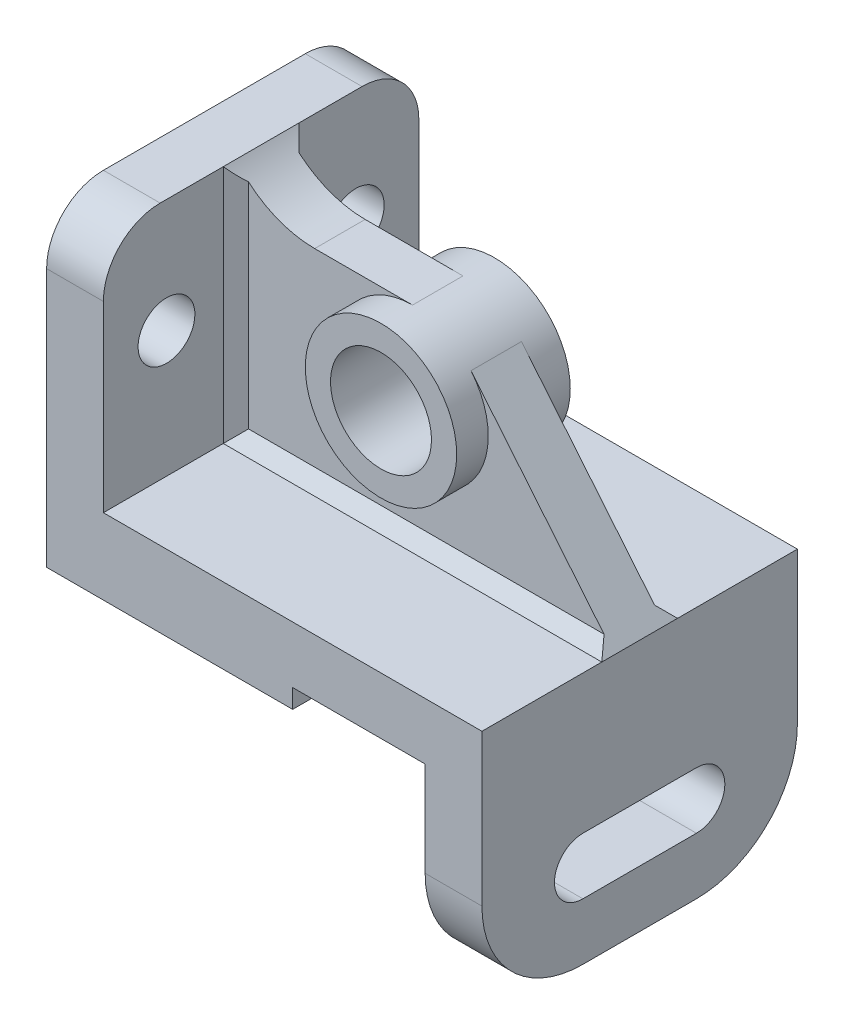
ISO-10303-21;
HEADER;
FILE_DESCRIPTION(('STEP AP214'),'2;1');
FILE_NAME('part.step','',(''),(''),'','','');
FILE_SCHEMA(('AUTOMOTIVE_DESIGN { 1 0 10303 214 1 1 1 1 }'));
ENDSEC;
DATA;
#1=APPLICATION_CONTEXT('core data for automotive mechanical design processes');
#2=APPLICATION_PROTOCOL_DEFINITION('international standard','automotive_design',2000,#1);
#3=PRODUCT_CONTEXT('',#1,'mechanical');
#4=PRODUCT('Part','Part','',(#3));
#5=PRODUCT_RELATED_PRODUCT_CATEGORY('part','',(#4));
#6=PRODUCT_DEFINITION_FORMATION('','',#4);
#7=PRODUCT_DEFINITION_CONTEXT('part definition',#1,'design');
#8=PRODUCT_DEFINITION('design','',#6,#7);
#9=PRODUCT_DEFINITION_SHAPE('','',#8);
#10=(LENGTH_UNIT() NAMED_UNIT(*) SI_UNIT(.MILLI.,.METRE.));
#11=(NAMED_UNIT(*) PLANE_ANGLE_UNIT() SI_UNIT($,.RADIAN.));
#12=(NAMED_UNIT(*) SI_UNIT($,.STERADIAN.) SOLID_ANGLE_UNIT());
#13=UNCERTAINTY_MEASURE_WITH_UNIT(LENGTH_MEASURE(1.E-05),#10,'distance_accuracy_value','');
#14=(GEOMETRIC_REPRESENTATION_CONTEXT(3) GLOBAL_UNCERTAINTY_ASSIGNED_CONTEXT((#13)) GLOBAL_UNIT_ASSIGNED_CONTEXT((#10,
#11,#12)) REPRESENTATION_CONTEXT('',''));
#15=CARTESIAN_POINT('',(0.,0.,0.));
#16=DIRECTION('',(0.,0.,1.));
#17=DIRECTION('',(1.,0.,0.));
#18=AXIS2_PLACEMENT_3D('',#15,#16,#17);
#19=CARTESIAN_POINT('',(9.,12.,25.));
#20=DIRECTION('',(0.,-1.,0.));
#21=DIRECTION('',(1.,0.,0.));
#22=AXIS2_PLACEMENT_3D('',#19,#20,#21);
#23=PLANE('',#22);
#24=DIRECTION('',(0.,0.,-1.));
#25=VECTOR('',#24,1.);
#26=CARTESIAN_POINT('',(69.,12.,25.));
#27=LINE('',#26,#25);
#28=CARTESIAN_POINT('',(69.,12.,25.));
#29=VERTEX_POINT('',#28);
#30=CARTESIAN_POINT('',(69.,12.,6.));
#31=VERTEX_POINT('',#30);
#32=EDGE_CURVE('E354',#29,#31,#27,.T.);
#33=ORIENTED_EDGE('',*,*,#32,.T.);
#34=DIRECTION('',(-1.,0.,0.));
#35=VECTOR('',#34,1.);
#36=CARTESIAN_POINT('',(9.,12.,6.));
#37=LINE('',#36,#35);
#38=CARTESIAN_POINT('',(9.,12.,6.));
#39=VERTEX_POINT('',#38);
#40=EDGE_CURVE('E425',#31,#39,#37,.T.);
#41=ORIENTED_EDGE('',*,*,#40,.T.);
#42=DIRECTION('',(0.,0.,-1.));
#43=VECTOR('',#42,1.);
#44=CARTESIAN_POINT('',(9.,12.,25.));
#45=LINE('',#44,#43);
#46=CARTESIAN_POINT('',(9.,12.,25.));
#47=VERTEX_POINT('',#46);
#48=EDGE_CURVE('E351',#47,#39,#45,.T.);
#49=ORIENTED_EDGE('',*,*,#48,.F.);
#50=DIRECTION('',(-1.,0.,0.));
#51=VECTOR('',#50,1.);
#52=CARTESIAN_POINT('',(9.,12.,25.));
#53=LINE('',#52,#51);
#54=EDGE_CURVE('E313',#29,#47,#53,.T.);
#55=ORIENTED_EDGE('',*,*,#54,.F.);
#56=EDGE_LOOP('',(#33,#41,#49,#55));
#57=FACE_BOUND('',#56,.T.);
#58=ADVANCED_FACE('F41',(#57),#23,.F.);
#59=CARTESIAN_POINT('',(9.,50.,25.));
#60=DIRECTION('',(-1.,0.,0.));
#61=DIRECTION('',(0.,-1.,0.));
#62=AXIS2_PLACEMENT_3D('',#59,#60,#61);
#63=PLANE('',#62);
#64=CARTESIAN_POINT('',(9.,32.,15.));
#65=DIRECTION('',(1.,0.,0.));
#66=DIRECTION('',(0.,1.,0.));
#67=AXIS2_PLACEMENT_3D('',#64,#65,#66);
#68=CIRCLE('',#67,4.5);
#69=CARTESIAN_POINT('',(9.,36.5,15.));
#70=VERTEX_POINT('',#69);
#71=EDGE_CURVE('E291',#70,#70,#68,.T.);
#72=ORIENTED_EDGE('',*,*,#71,.F.);
#73=EDGE_LOOP('',(#72));
#74=FACE_BOUND('',#73,.T.);
#75=ORIENTED_EDGE('',*,*,#48,.T.);
#76=DIRECTION('',(0.,1.,0.));
#77=VECTOR('',#76,1.);
#78=CARTESIAN_POINT('',(9.,50.,6.));
#79=LINE('',#78,#77);
#80=CARTESIAN_POINT('',(9.,50.,6.));
#81=VERTEX_POINT('',#80);
#82=EDGE_CURVE('E428',#39,#81,#79,.T.);
#83=ORIENTED_EDGE('',*,*,#82,.T.);
#84=DIRECTION('',(0.,0.,-1.));
#85=VECTOR('',#84,1.);
#86=CARTESIAN_POINT('',(9.,50.,25.));
#87=LINE('',#86,#85);
#88=CARTESIAN_POINT('',(9.,50.,16.));
#89=VERTEX_POINT('',#88);
#90=EDGE_CURVE('E349',#89,#81,#87,.T.);
#91=ORIENTED_EDGE('',*,*,#90,.F.);
#92=CARTESIAN_POINT('',(9.,41.,16.));
#93=DIRECTION('',(-1.,0.,0.));
#94=DIRECTION('',(0.,-1.,0.));
#95=AXIS2_PLACEMENT_3D('',#92,#93,#94);
#96=CIRCLE('',#95,9.);
#97=CARTESIAN_POINT('',(9.,41.,25.));
#98=VERTEX_POINT('',#97);
#99=EDGE_CURVE('E384',#89,#98,#96,.F.);
#100=ORIENTED_EDGE('',*,*,#99,.T.);
#101=DIRECTION('',(0.,1.,0.));
#102=VECTOR('',#101,1.);
#103=CARTESIAN_POINT('',(9.,50.,25.));
#104=LINE('',#103,#102);
#105=EDGE_CURVE('E317',#47,#98,#104,.T.);
#106=ORIENTED_EDGE('',*,*,#105,.F.);
#107=EDGE_LOOP('',(#75,#83,#91,#100,#106));
#108=FACE_BOUND('',#107,.T.);
#109=ADVANCED_FACE('F459',(#74,#108),#63,.F.);
#110=CARTESIAN_POINT('',(39.,0.,25.));
#111=DIRECTION('',(0.,1.,0.));
#112=DIRECTION('',(-1.,0.,0.));
#113=AXIS2_PLACEMENT_3D('',#110,#111,#112);
#114=PLANE('',#113);
#115=DIRECTION('',(1.,0.,0.));
#116=VECTOR('',#115,1.);
#117=CARTESIAN_POINT('',(39.,0.,-25.));
#118=LINE('',#117,#116);
#119=CARTESIAN_POINT('',(0.,0.,-25.));
#120=VERTEX_POINT('',#119);
#121=CARTESIAN_POINT('',(39.,0.,-25.));
#122=VERTEX_POINT('',#121);
#123=EDGE_CURVE('E292',#120,#122,#118,.T.);
#124=ORIENTED_EDGE('',*,*,#123,.T.);
#125=DIRECTION('',(0.,0.,-1.));
#126=VECTOR('',#125,1.);
#127=CARTESIAN_POINT('',(39.,0.,25.));
#128=LINE('',#127,#126);
#129=CARTESIAN_POINT('',(39.,0.,25.));
#130=VERTEX_POINT('',#129);
#131=EDGE_CURVE('E367',#130,#122,#128,.T.);
#132=ORIENTED_EDGE('',*,*,#131,.F.);
#133=DIRECTION('',(1.,0.,0.));
#134=VECTOR('',#133,1.);
#135=CARTESIAN_POINT('',(39.,0.,25.));
#136=LINE('',#135,#134);
#137=CARTESIAN_POINT('',(0.,0.,25.));
#138=VERTEX_POINT('',#137);
#139=EDGE_CURVE('E301',#138,#130,#136,.T.);
#140=ORIENTED_EDGE('',*,*,#139,.F.);
#141=DIRECTION('',(0.,0.,-1.));
#142=VECTOR('',#141,1.);
#143=CARTESIAN_POINT('',(0.,0.,25.));
#144=LINE('',#143,#142);
#145=EDGE_CURVE('E322',#138,#120,#144,.T.);
#146=ORIENTED_EDGE('',*,*,#145,.T.);
#147=EDGE_LOOP('',(#124,#132,#140,#146));
#148=FACE_BOUND('',#147,.T.);
#149=ADVANCED_FACE('F523',(#148),#114,.F.);
#150=CARTESIAN_POINT('',(39.,3.,25.));
#151=DIRECTION('',(-1.,0.,0.));
#152=DIRECTION('',(0.,0.,1.));
#153=AXIS2_PLACEMENT_3D('',#150,#151,#152);
#154=PLANE('',#153);
#155=DIRECTION('',(0.,1.,0.));
#156=VECTOR('',#155,1.);
#157=CARTESIAN_POINT('',(39.,3.,-25.));
#158=LINE('',#157,#156);
#159=CARTESIAN_POINT('',(39.,3.,-25.));
#160=VERTEX_POINT('',#159);
#161=EDGE_CURVE('E321',#122,#160,#158,.T.);
#162=ORIENTED_EDGE('',*,*,#161,.T.);
#163=DIRECTION('',(0.,0.,-1.));
#164=VECTOR('',#163,1.);
#165=CARTESIAN_POINT('',(39.,3.,25.));
#166=LINE('',#165,#164);
#167=CARTESIAN_POINT('',(39.,3.,25.));
#168=VERTEX_POINT('',#167);
#169=EDGE_CURVE('E366',#168,#160,#166,.T.);
#170=ORIENTED_EDGE('',*,*,#169,.F.);
#171=DIRECTION('',(0.,1.,0.));
#172=VECTOR('',#171,1.);
#173=CARTESIAN_POINT('',(39.,3.,25.));
#174=LINE('',#173,#172);
#175=EDGE_CURVE('E302',#130,#168,#174,.T.);
#176=ORIENTED_EDGE('',*,*,#175,.F.);
#177=ORIENTED_EDGE('',*,*,#131,.T.);
#178=EDGE_LOOP('',(#162,#170,#176,#177));
#179=FACE_BOUND('',#178,.T.);
#180=ADVANCED_FACE('F700',(#179),#154,.F.);
#181=CARTESIAN_POINT('',(60.,3.,25.));
#182=DIRECTION('',(0.,1.,0.));
#183=DIRECTION('',(-1.,0.,0.));
#184=AXIS2_PLACEMENT_3D('',#181,#182,#183);
#185=PLANE('',#184);
#186=DIRECTION('',(1.,0.,0.));
#187=VECTOR('',#186,1.);
#188=CARTESIAN_POINT('',(60.,3.,-25.));
#189=LINE('',#188,#187);
#190=CARTESIAN_POINT('',(60.,3.,-25.));
#191=VERTEX_POINT('',#190);
#192=EDGE_CURVE('E328',#160,#191,#189,.T.);
#193=ORIENTED_EDGE('',*,*,#192,.T.);
#194=DIRECTION('',(0.,0.,-1.));
#195=VECTOR('',#194,1.);
#196=CARTESIAN_POINT('',(60.,3.,25.));
#197=LINE('',#196,#195);
#198=CARTESIAN_POINT('',(60.,3.,25.));
#199=VERTEX_POINT('',#198);
#200=EDGE_CURVE('E361',#199,#191,#197,.T.);
#201=ORIENTED_EDGE('',*,*,#200,.F.);
#202=DIRECTION('',(1.,0.,0.));
#203=VECTOR('',#202,1.);
#204=CARTESIAN_POINT('',(60.,3.,25.));
#205=LINE('',#204,#203);
#206=EDGE_CURVE('E310',#168,#199,#205,.T.);
#207=ORIENTED_EDGE('',*,*,#206,.F.);
#208=ORIENTED_EDGE('',*,*,#169,.T.);
#209=EDGE_LOOP('',(#193,#201,#207,#208));
#210=FACE_BOUND('',#209,.T.);
#211=ADVANCED_FACE('F701',(#210),#185,.F.);
#212=CARTESIAN_POINT('',(60.,-28.,25.));
#213=DIRECTION('',(1.,0.,0.));
#214=DIRECTION('',(0.,0.,-1.));
#215=AXIS2_PLACEMENT_3D('',#212,#213,#214);
#216=PLANE('',#215);
#217=DIRECTION('',(0.,0.,1.));
#218=VECTOR('',#217,1.);
#219=CARTESIAN_POINT('',(60.,-10.,9.));
#220=LINE('',#219,#218);
#221=CARTESIAN_POINT('',(60.,-10.,-9.));
#222=VERTEX_POINT('',#221);
#223=CARTESIAN_POINT('',(60.,-10.,9.));
#224=VERTEX_POINT('',#223);
#225=EDGE_CURVE('E256',#222,#224,#220,.T.);
#226=ORIENTED_EDGE('',*,*,#225,.T.);
#227=CARTESIAN_POINT('',(60.,-14.5,9.));
#228=DIRECTION('',(1.,0.,0.));
#229=DIRECTION('',(0.,0.,-1.));
#230=AXIS2_PLACEMENT_3D('',#227,#228,#229);
#231=CIRCLE('',#230,4.5);
#232=CARTESIAN_POINT('',(60.,-19.,9.));
#233=VERTEX_POINT('',#232);
#234=EDGE_CURVE('E264',#233,#224,#231,.F.);
#235=ORIENTED_EDGE('',*,*,#234,.F.);
#236=DIRECTION('',(0.,0.,1.));
#237=VECTOR('',#236,1.);
#238=CARTESIAN_POINT('',(60.,-19.,9.));
#239=LINE('',#238,#237);
#240=CARTESIAN_POINT('',(60.,-19.,-9.));
#241=VERTEX_POINT('',#240);
#242=EDGE_CURVE('E276',#241,#233,#239,.T.);
#243=ORIENTED_EDGE('',*,*,#242,.F.);
#244=CARTESIAN_POINT('',(60.,-14.5,-9.));
#245=DIRECTION('',(1.,0.,0.));
#246=DIRECTION('',(0.,0.,-1.));
#247=AXIS2_PLACEMENT_3D('',#244,#245,#246);
#248=CIRCLE('',#247,4.5);
#249=EDGE_CURVE('E260',#222,#241,#248,.F.);
#250=ORIENTED_EDGE('',*,*,#249,.F.);
#251=EDGE_LOOP('',(#226,#235,#243,#250));
#252=FACE_BOUND('',#251,.T.);
#253=DIRECTION('',(0.,-1.,0.));
#254=VECTOR('',#253,1.);
#255=CARTESIAN_POINT('',(60.,-28.,-25.));
#256=LINE('',#255,#254);
#257=CARTESIAN_POINT('',(60.,-12.,-25.));
#258=VERTEX_POINT('',#257);
#259=EDGE_CURVE('E327',#191,#258,#256,.T.);
#260=ORIENTED_EDGE('',*,*,#259,.T.);
#261=CARTESIAN_POINT('',(60.,-12.,-9.));
#262=DIRECTION('',(1.,0.,0.));
#263=DIRECTION('',(0.,0.,-1.));
#264=AXIS2_PLACEMENT_3D('',#261,#262,#263);
#265=CIRCLE('',#264,16.);
#266=CARTESIAN_POINT('',(60.,-28.,-9.));
#267=VERTEX_POINT('',#266);
#268=EDGE_CURVE('E404',#258,#267,#265,.F.);
#269=ORIENTED_EDGE('',*,*,#268,.T.);
#270=DIRECTION('',(0.,0.,-1.));
#271=VECTOR('',#270,1.);
#272=CARTESIAN_POINT('',(60.,-28.,25.));
#273=LINE('',#272,#271);
#274=CARTESIAN_POINT('',(60.,-28.,9.));
#275=VERTEX_POINT('',#274);
#276=EDGE_CURVE('E359',#275,#267,#273,.T.);
#277=ORIENTED_EDGE('',*,*,#276,.F.);
#278=CARTESIAN_POINT('',(60.,-12.,9.));
#279=DIRECTION('',(1.,0.,0.));
#280=DIRECTION('',(0.,0.,-1.));
#281=AXIS2_PLACEMENT_3D('',#278,#279,#280);
#282=CIRCLE('',#281,16.);
#283=CARTESIAN_POINT('',(60.,-12.,25.));
#284=VERTEX_POINT('',#283);
#285=EDGE_CURVE('E405',#275,#284,#282,.F.);
#286=ORIENTED_EDGE('',*,*,#285,.T.);
#287=DIRECTION('',(0.,-1.,0.));
#288=VECTOR('',#287,1.);
#289=CARTESIAN_POINT('',(60.,-28.,25.));
#290=LINE('',#289,#288);
#291=EDGE_CURVE('E307',#199,#284,#290,.T.);
#292=ORIENTED_EDGE('',*,*,#291,.F.);
#293=ORIENTED_EDGE('',*,*,#200,.T.);
#294=EDGE_LOOP('',(#260,#269,#277,#286,#292,#293));
#295=FACE_BOUND('',#294,.T.);
#296=ADVANCED_FACE('F704',(#252,#295),#216,.F.);
#297=CARTESIAN_POINT('',(69.,-28.,25.));
#298=DIRECTION('',(0.,1.,0.));
#299=DIRECTION('',(0.,0.,1.));
#300=AXIS2_PLACEMENT_3D('',#297,#298,#299);
#301=PLANE('',#300);
#302=ORIENTED_EDGE('',*,*,#276,.T.);
#303=DIRECTION('',(1.,0.,0.));
#304=VECTOR('',#303,1.);
#305=CARTESIAN_POINT('',(69.,-28.,-9.));
#306=LINE('',#305,#304);
#307=CARTESIAN_POINT('',(69.,-28.,-9.));
#308=VERTEX_POINT('',#307);
#309=EDGE_CURVE('E392',#267,#308,#306,.T.);
#310=ORIENTED_EDGE('',*,*,#309,.T.);
#311=DIRECTION('',(0.,0.,-1.));
#312=VECTOR('',#311,1.);
#313=CARTESIAN_POINT('',(69.,-28.,25.));
#314=LINE('',#313,#312);
#315=CARTESIAN_POINT('',(69.,-28.,9.));
#316=VERTEX_POINT('',#315);
#317=EDGE_CURVE('E357',#316,#308,#314,.T.);
#318=ORIENTED_EDGE('',*,*,#317,.F.);
#319=DIRECTION('',(1.,0.,0.));
#320=VECTOR('',#319,1.);
#321=CARTESIAN_POINT('',(69.,-28.,9.));
#322=LINE('',#321,#320);
#323=EDGE_CURVE('E393',#316,#275,#322,.F.);
#324=ORIENTED_EDGE('',*,*,#323,.T.);
#325=EDGE_LOOP('',(#302,#310,#318,#324));
#326=FACE_BOUND('',#325,.T.);
#327=ADVANCED_FACE('F534',(#326),#301,.F.);
#328=CARTESIAN_POINT('',(69.,12.,25.));
#329=DIRECTION('',(-1.,0.,0.));
#330=DIRECTION('',(0.,0.,1.));
#331=AXIS2_PLACEMENT_3D('',#328,#329,#330);
#332=PLANE('',#331);
#333=DIRECTION('',(0.,0.,-1.));
#334=VECTOR('',#333,1.);
#335=CARTESIAN_POINT('',(69.,-19.,9.));
#336=LINE('',#335,#334);
#337=CARTESIAN_POINT('',(69.,-19.,9.));
#338=VERTEX_POINT('',#337);
#339=CARTESIAN_POINT('',(69.,-19.,-9.));
#340=VERTEX_POINT('',#339);
#341=EDGE_CURVE('E270',#338,#340,#336,.T.);
#342=ORIENTED_EDGE('',*,*,#341,.F.);
#343=CARTESIAN_POINT('',(69.,-14.5,9.));
#344=DIRECTION('',(1.,0.,0.));
#345=DIRECTION('',(0.,0.,-1.));
#346=AXIS2_PLACEMENT_3D('',#343,#344,#345);
#347=CIRCLE('',#346,4.5);
#348=CARTESIAN_POINT('',(69.,-10.,9.));
#349=VERTEX_POINT('',#348);
#350=EDGE_CURVE('E261',#349,#338,#347,.T.);
#351=ORIENTED_EDGE('',*,*,#350,.F.);
#352=DIRECTION('',(0.,0.,-1.));
#353=VECTOR('',#352,1.);
#354=CARTESIAN_POINT('',(69.,-10.,9.));
#355=LINE('',#354,#353);
#356=CARTESIAN_POINT('',(69.,-10.,-9.));
#357=VERTEX_POINT('',#356);
#358=EDGE_CURVE('E271',#349,#357,#355,.T.);
#359=ORIENTED_EDGE('',*,*,#358,.T.);
#360=CARTESIAN_POINT('',(69.,-14.5,-9.));
#361=DIRECTION('',(1.,0.,0.));
#362=DIRECTION('',(0.,0.,-1.));
#363=AXIS2_PLACEMENT_3D('',#360,#361,#362);
#364=CIRCLE('',#363,4.5);
#365=EDGE_CURVE('E269',#340,#357,#364,.T.);
#366=ORIENTED_EDGE('',*,*,#365,.F.);
#367=EDGE_LOOP('',(#342,#351,#359,#366));
#368=FACE_BOUND('',#367,.T.);
#369=ORIENTED_EDGE('',*,*,#317,.T.);
#370=CARTESIAN_POINT('',(69.,-12.,-9.));
#371=DIRECTION('',(-1.,0.,0.));
#372=DIRECTION('',(0.,0.,1.));
#373=AXIS2_PLACEMENT_3D('',#370,#371,#372);
#374=CIRCLE('',#373,16.);
#375=CARTESIAN_POINT('',(69.,-12.,-25.));
#376=VERTEX_POINT('',#375);
#377=EDGE_CURVE('E398',#308,#376,#374,.F.);
#378=ORIENTED_EDGE('',*,*,#377,.T.);
#379=DIRECTION('',(0.,1.,0.));
#380=VECTOR('',#379,1.);
#381=CARTESIAN_POINT('',(69.,12.,-25.));
#382=LINE('',#381,#380);
#383=CARTESIAN_POINT('',(69.,12.,-25.));
#384=VERTEX_POINT('',#383);
#385=EDGE_CURVE('E331',#376,#384,#382,.T.);
#386=ORIENTED_EDGE('',*,*,#385,.T.);
#387=CARTESIAN_POINT('',(69.,12.,-6.00000000000002));
#388=VERTEX_POINT('',#387);
#389=EDGE_CURVE('E352',#388,#384,#27,.T.);
#390=ORIENTED_EDGE('',*,*,#389,.F.);
#391=DIRECTION('',(0.,0.,-1.));
#392=VECTOR('',#391,1.);
#393=CARTESIAN_POINT('',(69.,12.,4.));
#394=LINE('',#393,#392);
#395=EDGE_CURVE('E58',#31,#388,#394,.T.);
#396=ORIENTED_EDGE('',*,*,#395,.F.);
#397=ORIENTED_EDGE('',*,*,#32,.F.);
#398=DIRECTION('',(0.,1.,0.));
#399=VECTOR('',#398,1.);
#400=CARTESIAN_POINT('',(69.,12.,25.));
#401=LINE('',#400,#399);
#402=CARTESIAN_POINT('',(69.,-12.,25.));
#403=VERTEX_POINT('',#402);
#404=EDGE_CURVE('E315',#403,#29,#401,.T.);
#405=ORIENTED_EDGE('',*,*,#404,.F.);
#406=CARTESIAN_POINT('',(69.,-12.,9.));
#407=DIRECTION('',(-1.,0.,0.));
#408=DIRECTION('',(0.,0.,1.));
#409=AXIS2_PLACEMENT_3D('',#406,#407,#408);
#410=CIRCLE('',#409,16.);
#411=EDGE_CURVE('E396',#403,#316,#410,.F.);
#412=ORIENTED_EDGE('',*,*,#411,.T.);
#413=EDGE_LOOP('',(#369,#378,#386,#390,#396,#397,#405,#412));
#414=FACE_BOUND('',#413,.T.);
#415=ADVANCED_FACE('F530',(#368,#414),#332,.F.);
#416=CARTESIAN_POINT('',(9.,12.,-6.00000000000002));
#417=VERTEX_POINT('',#416);
#418=CARTESIAN_POINT('',(9.,12.,-25.));
#419=VERTEX_POINT('',#418);
#420=EDGE_CURVE('E346',#417,#419,#45,.T.);
#421=ORIENTED_EDGE('',*,*,#420,.F.);
#422=DIRECTION('',(1.,0.,0.));
#423=VECTOR('',#422,1.);
#424=CARTESIAN_POINT('',(9.,12.,-6.00000000000002));
#425=LINE('',#424,#423);
#426=EDGE_CURVE('E416',#417,#388,#425,.T.);
#427=ORIENTED_EDGE('',*,*,#426,.T.);
#428=ORIENTED_EDGE('',*,*,#389,.T.);
#429=DIRECTION('',(-1.,0.,0.));
#430=VECTOR('',#429,1.);
#431=CARTESIAN_POINT('',(9.,12.,-25.));
#432=LINE('',#431,#430);
#433=EDGE_CURVE('E332',#384,#419,#432,.T.);
#434=ORIENTED_EDGE('',*,*,#433,.T.);
#435=EDGE_LOOP('',(#421,#427,#428,#434));
#436=FACE_BOUND('',#435,.T.);
#437=ADVANCED_FACE('F517',(#436),#23,.F.);
#438=CARTESIAN_POINT('',(9.,32.,-15.));
#439=DIRECTION('',(1.,0.,0.));
#440=DIRECTION('',(0.,1.,0.));
#441=AXIS2_PLACEMENT_3D('',#438,#439,#440);
#442=CIRCLE('',#441,4.50000000000001);
#443=CARTESIAN_POINT('',(9.,36.5,-15.));
#444=VERTEX_POINT('',#443);
#445=EDGE_CURVE('E298',#444,#444,#442,.T.);
#446=ORIENTED_EDGE('',*,*,#445,.F.);
#447=EDGE_LOOP('',(#446));
#448=FACE_BOUND('',#447,.T.);
#449=CARTESIAN_POINT('',(9.,50.,-6.00000000000002));
#450=VERTEX_POINT('',#449);
#451=CARTESIAN_POINT('',(9.,50.,-16.));
#452=VERTEX_POINT('',#451);
#453=EDGE_CURVE('E348',#450,#452,#87,.T.);
#454=ORIENTED_EDGE('',*,*,#453,.F.);
#455=DIRECTION('',(0.,-1.,0.));
#456=VECTOR('',#455,1.);
#457=CARTESIAN_POINT('',(9.,50.,-6.00000000000002));
#458=LINE('',#457,#456);
#459=EDGE_CURVE('E406',#450,#417,#458,.T.);
#460=ORIENTED_EDGE('',*,*,#459,.T.);
#461=ORIENTED_EDGE('',*,*,#420,.T.);
#462=DIRECTION('',(0.,1.,0.));
#463=VECTOR('',#462,1.);
#464=CARTESIAN_POINT('',(9.,50.,-25.));
#465=LINE('',#464,#463);
#466=CARTESIAN_POINT('',(9.,41.,-25.));
#467=VERTEX_POINT('',#466);
#468=EDGE_CURVE('E340',#419,#467,#465,.T.);
#469=ORIENTED_EDGE('',*,*,#468,.T.);
#470=CARTESIAN_POINT('',(9.,41.,-16.));
#471=DIRECTION('',(-1.,0.,0.));
#472=DIRECTION('',(0.,-1.,0.));
#473=AXIS2_PLACEMENT_3D('',#470,#471,#472);
#474=CIRCLE('',#473,9.);
#475=EDGE_CURVE('E383',#467,#452,#474,.F.);
#476=ORIENTED_EDGE('',*,*,#475,.T.);
#477=EDGE_LOOP('',(#454,#460,#461,#469,#476));
#478=FACE_BOUND('',#477,.T.);
#479=ADVANCED_FACE('F525',(#448,#478),#63,.F.);
#480=CARTESIAN_POINT('',(0.,50.,25.));
#481=DIRECTION('',(0.,-1.,0.));
#482=DIRECTION('',(0.,0.,-1.));
#483=AXIS2_PLACEMENT_3D('',#480,#481,#482);
#484=PLANE('',#483);
#485=ORIENTED_EDGE('',*,*,#90,.T.);
#486=DIRECTION('',(0.,0.,-1.));
#487=VECTOR('',#486,1.);
#488=CARTESIAN_POINT('',(9.,50.,4.));
#489=LINE('',#488,#487);
#490=EDGE_CURVE('E252',#81,#450,#489,.T.);
#491=ORIENTED_EDGE('',*,*,#490,.T.);
#492=ORIENTED_EDGE('',*,*,#453,.T.);
#493=DIRECTION('',(-1.,0.,0.));
#494=VECTOR('',#493,1.);
#495=CARTESIAN_POINT('',(0.,50.,-16.));
#496=LINE('',#495,#494);
#497=CARTESIAN_POINT('',(0.,50.,-16.));
#498=VERTEX_POINT('',#497);
#499=EDGE_CURVE('E372',#452,#498,#496,.T.);
#500=ORIENTED_EDGE('',*,*,#499,.T.);
#501=DIRECTION('',(0.,0.,-1.));
#502=VECTOR('',#501,1.);
#503=CARTESIAN_POINT('',(0.,50.,25.));
#504=LINE('',#503,#502);
#505=CARTESIAN_POINT('',(0.,50.,16.));
#506=VERTEX_POINT('',#505);
#507=EDGE_CURVE('E344',#506,#498,#504,.T.);
#508=ORIENTED_EDGE('',*,*,#507,.F.);
#509=DIRECTION('',(-1.,0.,0.));
#510=VECTOR('',#509,1.);
#511=CARTESIAN_POINT('',(0.,50.,16.));
#512=LINE('',#511,#510);
#513=EDGE_CURVE('E375',#506,#89,#512,.F.);
#514=ORIENTED_EDGE('',*,*,#513,.T.);
#515=EDGE_LOOP('',(#485,#491,#492,#500,#508,#514));
#516=FACE_BOUND('',#515,.T.);
#517=ADVANCED_FACE('F463',(#516),#484,.F.);
#518=CARTESIAN_POINT('',(0.,0.,25.));
#519=DIRECTION('',(1.,0.,0.));
#520=DIRECTION('',(0.,0.,-1.));
#521=AXIS2_PLACEMENT_3D('',#518,#519,#520);
#522=PLANE('',#521);
#523=CARTESIAN_POINT('',(0.,32.,15.));
#524=DIRECTION('',(1.,0.,0.));
#525=DIRECTION('',(0.,1.,0.));
#526=AXIS2_PLACEMENT_3D('',#523,#524,#525);
#527=CIRCLE('',#526,4.5);
#528=CARTESIAN_POINT('',(0.,36.5,15.));
#529=VERTEX_POINT('',#528);
#530=EDGE_CURVE('E287',#529,#529,#527,.T.);
#531=ORIENTED_EDGE('',*,*,#530,.T.);
#532=EDGE_LOOP('',(#531));
#533=FACE_BOUND('',#532,.T.);
#534=CARTESIAN_POINT('',(0.,32.,-15.));
#535=DIRECTION('',(1.,0.,0.));
#536=DIRECTION('',(0.,1.,0.));
#537=AXIS2_PLACEMENT_3D('',#534,#535,#536);
#538=CIRCLE('',#537,4.50000000000001);
#539=CARTESIAN_POINT('',(0.,36.5,-15.));
#540=VERTEX_POINT('',#539);
#541=EDGE_CURVE('E288',#540,#540,#538,.T.);
#542=ORIENTED_EDGE('',*,*,#541,.T.);
#543=EDGE_LOOP('',(#542));
#544=FACE_BOUND('',#543,.T.);
#545=ORIENTED_EDGE('',*,*,#507,.T.);
#546=CARTESIAN_POINT('',(0.,41.,-16.));
#547=DIRECTION('',(1.,0.,0.));
#548=DIRECTION('',(0.,0.,-1.));
#549=AXIS2_PLACEMENT_3D('',#546,#547,#548);
#550=CIRCLE('',#549,9.);
#551=CARTESIAN_POINT('',(0.,41.,-25.));
#552=VERTEX_POINT('',#551);
#553=EDGE_CURVE('E378',#498,#552,#550,.F.);
#554=ORIENTED_EDGE('',*,*,#553,.T.);
#555=DIRECTION('',(0.,-1.,0.));
#556=VECTOR('',#555,1.);
#557=CARTESIAN_POINT('',(0.,0.,-25.));
#558=LINE('',#557,#556);
#559=EDGE_CURVE('E304',#552,#120,#558,.T.);
#560=ORIENTED_EDGE('',*,*,#559,.T.);
#561=ORIENTED_EDGE('',*,*,#145,.F.);
#562=DIRECTION('',(0.,-1.,0.));
#563=VECTOR('',#562,1.);
#564=CARTESIAN_POINT('',(0.,0.,25.));
#565=LINE('',#564,#563);
#566=CARTESIAN_POINT('',(0.,41.,25.));
#567=VERTEX_POINT('',#566);
#568=EDGE_CURVE('E316',#567,#138,#565,.T.);
#569=ORIENTED_EDGE('',*,*,#568,.F.);
#570=CARTESIAN_POINT('',(0.,41.,16.));
#571=DIRECTION('',(1.,0.,0.));
#572=DIRECTION('',(0.,0.,-1.));
#573=AXIS2_PLACEMENT_3D('',#570,#571,#572);
#574=CIRCLE('',#573,9.);
#575=EDGE_CURVE('E380',#567,#506,#574,.F.);
#576=ORIENTED_EDGE('',*,*,#575,.T.);
#577=EDGE_LOOP('',(#545,#554,#560,#561,#569,#576));
#578=FACE_BOUND('',#577,.T.);
#579=ADVANCED_FACE('F581',(#533,#544,#578),#522,.F.);
#580=CARTESIAN_POINT('',(0.,0.,25.));
#581=DIRECTION('',(0.,0.,-1.));
#582=DIRECTION('',(-1.,0.,0.));
#583=AXIS2_PLACEMENT_3D('',#580,#581,#582);
#584=PLANE('',#583);
#585=ORIENTED_EDGE('',*,*,#291,.T.);
#586=DIRECTION('',(1.,0.,0.));
#587=VECTOR('',#586,1.);
#588=CARTESIAN_POINT('',(0.,-12.,25.));
#589=LINE('',#588,#587);
#590=EDGE_CURVE('E407',#284,#403,#589,.T.);
#591=ORIENTED_EDGE('',*,*,#590,.T.);
#592=ORIENTED_EDGE('',*,*,#404,.T.);
#593=ORIENTED_EDGE('',*,*,#54,.T.);
#594=ORIENTED_EDGE('',*,*,#105,.T.);
#595=DIRECTION('',(-1.,0.,0.));
#596=VECTOR('',#595,1.);
#597=CARTESIAN_POINT('',(0.,41.,25.));
#598=LINE('',#597,#596);
#599=EDGE_CURVE('E389',#98,#567,#598,.T.);
#600=ORIENTED_EDGE('',*,*,#599,.T.);
#601=ORIENTED_EDGE('',*,*,#568,.T.);
#602=ORIENTED_EDGE('',*,*,#139,.T.);
#603=ORIENTED_EDGE('',*,*,#175,.T.);
#604=ORIENTED_EDGE('',*,*,#206,.T.);
#605=EDGE_LOOP('',(#585,#591,#592,#593,#594,#600,#601,#602,#603,#604));
#606=FACE_BOUND('',#605,.T.);
#607=ADVANCED_FACE('F472',(#606),#584,.F.);
#608=CARTESIAN_POINT('',(0.,0.,-25.));
#609=DIRECTION('',(0.,0.,-1.));
#610=DIRECTION('',(-1.,0.,0.));
#611=AXIS2_PLACEMENT_3D('',#608,#609,#610);
#612=PLANE('',#611);
#613=ORIENTED_EDGE('',*,*,#385,.F.);
#614=DIRECTION('',(1.,0.,0.));
#615=VECTOR('',#614,1.);
#616=CARTESIAN_POINT('',(60.,-12.,-25.));
#617=LINE('',#616,#615);
#618=EDGE_CURVE('E399',#376,#258,#617,.F.);
#619=ORIENTED_EDGE('',*,*,#618,.T.);
#620=ORIENTED_EDGE('',*,*,#259,.F.);
#621=ORIENTED_EDGE('',*,*,#192,.F.);
#622=ORIENTED_EDGE('',*,*,#161,.F.);
#623=ORIENTED_EDGE('',*,*,#123,.F.);
#624=ORIENTED_EDGE('',*,*,#559,.F.);
#625=DIRECTION('',(-1.,0.,0.));
#626=VECTOR('',#625,1.);
#627=CARTESIAN_POINT('',(9.,41.,-25.));
#628=LINE('',#627,#626);
#629=EDGE_CURVE('E382',#552,#467,#628,.F.);
#630=ORIENTED_EDGE('',*,*,#629,.T.);
#631=ORIENTED_EDGE('',*,*,#468,.F.);
#632=ORIENTED_EDGE('',*,*,#433,.F.);
#633=EDGE_LOOP('',(#613,#619,#620,#621,#622,#623,#624,#630,#631,#632));
#634=FACE_BOUND('',#633,.T.);
#635=ADVANCED_FACE('F584',(#634),#612,.T.);
#636=CARTESIAN_POINT('',(0.,41.,-16.));
#637=DIRECTION('',(1.,0.,0.));
#638=DIRECTION('',(0.,0.,-1.));
#639=AXIS2_PLACEMENT_3D('',#636,#637,#638);
#640=CYLINDRICAL_SURFACE('',#639,9.);
#641=ORIENTED_EDGE('',*,*,#475,.F.);
#642=ORIENTED_EDGE('',*,*,#629,.F.);
#643=ORIENTED_EDGE('',*,*,#553,.F.);
#644=ORIENTED_EDGE('',*,*,#499,.F.);
#645=EDGE_LOOP('',(#641,#642,#643,#644));
#646=FACE_BOUND('',#645,.T.);
#647=ADVANCED_FACE('F589',(#646),#640,.T.);
#648=CARTESIAN_POINT('',(0.,41.,16.));
#649=DIRECTION('',(-1.,0.,0.));
#650=DIRECTION('',(0.,0.,1.));
#651=AXIS2_PLACEMENT_3D('',#648,#649,#650);
#652=CYLINDRICAL_SURFACE('',#651,9.);
#653=ORIENTED_EDGE('',*,*,#99,.F.);
#654=ORIENTED_EDGE('',*,*,#513,.F.);
#655=ORIENTED_EDGE('',*,*,#575,.F.);
#656=ORIENTED_EDGE('',*,*,#599,.F.);
#657=EDGE_LOOP('',(#653,#654,#655,#656));
#658=FACE_BOUND('',#657,.T.);
#659=ADVANCED_FACE('F466',(#658),#652,.T.);
#660=CARTESIAN_POINT('',(69.,-12.,-9.));
#661=DIRECTION('',(-1.,0.,0.));
#662=DIRECTION('',(0.,0.,1.));
#663=AXIS2_PLACEMENT_3D('',#660,#661,#662);
#664=CYLINDRICAL_SURFACE('',#663,16.);
#665=ORIENTED_EDGE('',*,*,#268,.F.);
#666=ORIENTED_EDGE('',*,*,#618,.F.);
#667=ORIENTED_EDGE('',*,*,#377,.F.);
#668=ORIENTED_EDGE('',*,*,#309,.F.);
#669=EDGE_LOOP('',(#665,#666,#667,#668));
#670=FACE_BOUND('',#669,.T.);
#671=ADVANCED_FACE('F684',(#670),#664,.T.);
#672=CARTESIAN_POINT('',(0.,-12.,9.));
#673=DIRECTION('',(1.,0.,0.));
#674=DIRECTION('',(0.,0.,-1.));
#675=AXIS2_PLACEMENT_3D('',#672,#673,#674);
#676=CYLINDRICAL_SURFACE('',#675,16.);
#677=ORIENTED_EDGE('',*,*,#285,.F.);
#678=ORIENTED_EDGE('',*,*,#323,.F.);
#679=ORIENTED_EDGE('',*,*,#411,.F.);
#680=ORIENTED_EDGE('',*,*,#590,.F.);
#681=EDGE_LOOP('',(#677,#678,#679,#680));
#682=FACE_BOUND('',#681,.T.);
#683=ADVANCED_FACE('F576',(#682),#676,.T.);
#684=CARTESIAN_POINT('',(0.,32.,-15.));
#685=DIRECTION('',(1.,0.,0.));
#686=DIRECTION('',(0.,1.,0.));
#687=AXIS2_PLACEMENT_3D('',#684,#685,#686);
#688=CYLINDRICAL_SURFACE('',#687,4.50000000000001);
#689=ORIENTED_EDGE('',*,*,#541,.F.);
#690=EDGE_LOOP('',(#689));
#691=FACE_BOUND('',#690,.T.);
#692=ORIENTED_EDGE('',*,*,#445,.T.);
#693=EDGE_LOOP('',(#692));
#694=FACE_BOUND('',#693,.T.);
#695=ADVANCED_FACE('F574',(#691,#694),#688,.F.);
#696=CARTESIAN_POINT('',(0.,32.,15.));
#697=DIRECTION('',(1.,0.,0.));
#698=DIRECTION('',(0.,1.,0.));
#699=AXIS2_PLACEMENT_3D('',#696,#697,#698);
#700=CYLINDRICAL_SURFACE('',#699,4.5);
#701=ORIENTED_EDGE('',*,*,#530,.F.);
#702=EDGE_LOOP('',(#701));
#703=FACE_BOUND('',#702,.T.);
#704=ORIENTED_EDGE('',*,*,#71,.T.);
#705=EDGE_LOOP('',(#704));
#706=FACE_BOUND('',#705,.T.);
#707=ADVANCED_FACE('F571',(#703,#706),#700,.F.);
#708=CARTESIAN_POINT('',(-0.001000000000001,-14.5,9.));
#709=DIRECTION('',(1.,0.,0.));
#710=DIRECTION('',(0.,0.,-1.));
#711=AXIS2_PLACEMENT_3D('',#708,#709,#710);
#712=CYLINDRICAL_SURFACE('',#711,4.5);
#713=ORIENTED_EDGE('',*,*,#234,.T.);
#714=DIRECTION('',(1.,0.,0.));
#715=VECTOR('',#714,1.);
#716=CARTESIAN_POINT('',(-0.001000000000001,-10.,9.));
#717=LINE('',#716,#715);
#718=EDGE_CURVE('E280',#224,#349,#717,.T.);
#719=ORIENTED_EDGE('',*,*,#718,.T.);
#720=ORIENTED_EDGE('',*,*,#350,.T.);
#721=DIRECTION('',(1.,0.,0.));
#722=VECTOR('',#721,1.);
#723=CARTESIAN_POINT('',(-0.001000000000001,-19.,9.));
#724=LINE('',#723,#722);
#725=EDGE_CURVE('E277',#233,#338,#724,.T.);
#726=ORIENTED_EDGE('',*,*,#725,.F.);
#727=EDGE_LOOP('',(#713,#719,#720,#726));
#728=FACE_BOUND('',#727,.T.);
#729=ADVANCED_FACE('F561',(#728),#712,.F.);
#730=CARTESIAN_POINT('',(-0.001000000000001,-10.,9.));
#731=DIRECTION('',(0.,-1.,0.));
#732=DIRECTION('',(0.,0.,-1.));
#733=AXIS2_PLACEMENT_3D('',#730,#731,#732);
#734=PLANE('',#733);
#735=DIRECTION('',(1.,0.,0.));
#736=VECTOR('',#735,1.);
#737=CARTESIAN_POINT('',(-0.001000000000001,-10.,-9.));
#738=LINE('',#737,#736);
#739=EDGE_CURVE('E278',#222,#357,#738,.T.);
#740=ORIENTED_EDGE('',*,*,#739,.T.);
#741=ORIENTED_EDGE('',*,*,#358,.F.);
#742=ORIENTED_EDGE('',*,*,#718,.F.);
#743=ORIENTED_EDGE('',*,*,#225,.F.);
#744=EDGE_LOOP('',(#740,#741,#742,#743));
#745=FACE_BOUND('',#744,.T.);
#746=ADVANCED_FACE('F560',(#745),#734,.T.);
#747=CARTESIAN_POINT('',(-0.001000000000001,-14.5,-9.));
#748=DIRECTION('',(1.,0.,0.));
#749=DIRECTION('',(0.,0.,-1.));
#750=AXIS2_PLACEMENT_3D('',#747,#748,#749);
#751=CYLINDRICAL_SURFACE('',#750,4.5);
#752=ORIENTED_EDGE('',*,*,#249,.T.);
#753=DIRECTION('',(1.,0.,0.));
#754=VECTOR('',#753,1.);
#755=CARTESIAN_POINT('',(-0.001000000000001,-19.,-9.));
#756=LINE('',#755,#754);
#757=EDGE_CURVE('E284',#241,#340,#756,.T.);
#758=ORIENTED_EDGE('',*,*,#757,.T.);
#759=ORIENTED_EDGE('',*,*,#365,.T.);
#760=ORIENTED_EDGE('',*,*,#739,.F.);
#761=EDGE_LOOP('',(#752,#758,#759,#760));
#762=FACE_BOUND('',#761,.T.);
#763=ADVANCED_FACE('F557',(#762),#751,.F.);
#764=CARTESIAN_POINT('',(-0.001000000000001,-19.,9.));
#765=DIRECTION('',(0.,-1.,0.));
#766=DIRECTION('',(0.,0.,-1.));
#767=AXIS2_PLACEMENT_3D('',#764,#765,#766);
#768=PLANE('',#767);
#769=ORIENTED_EDGE('',*,*,#242,.T.);
#770=ORIENTED_EDGE('',*,*,#725,.T.);
#771=ORIENTED_EDGE('',*,*,#341,.T.);
#772=ORIENTED_EDGE('',*,*,#757,.F.);
#773=EDGE_LOOP('',(#769,#770,#771,#772));
#774=FACE_BOUND('',#773,.T.);
#775=ADVANCED_FACE('F558',(#774),#768,.F.);
#776=CARTESIAN_POINT('',(69.,12.,4.));
#777=DIRECTION('',(-0.772150107303324,-0.635440171685317,0.));
#778=DIRECTION('',(0.635440171685317,-0.772150107303324,0.));
#779=AXIS2_PLACEMENT_3D('',#776,#777,#778);
#780=PLANE('',#779);
#781=ORIENTED_EDGE('',*,*,#395,.T.);
#782=DIRECTION('',(-0.502954694135508,0.611161425339921,0.61116142533993));
#783=VECTOR('',#782,1.);
#784=CARTESIAN_POINT('',(65.9261349225073,15.7351828782353,-2.26481712176466));
#785=LINE('',#784,#783);
#786=CARTESIAN_POINT('',(67.3541019662497,14.,-4.));
#787=VERTEX_POINT('',#786);
#788=EDGE_CURVE('E435',#388,#787,#785,.T.);
#789=ORIENTED_EDGE('',*,*,#788,.T.);
#790=DIRECTION('',(-0.635440171685317,0.772150107303324,0.));
#791=VECTOR('',#790,1.);
#792=CARTESIAN_POINT('',(69.,12.,-4.));
#793=LINE('',#792,#791);
#794=CARTESIAN_POINT('',(46.2658012876399,39.6252820602238,-4.));
#795=VERTEX_POINT('',#794);
#796=EDGE_CURVE('E243',#787,#795,#793,.T.);
#797=ORIENTED_EDGE('',*,*,#796,.T.);
#798=DIRECTION('',(0.,0.,-1.));
#799=VECTOR('',#798,1.);
#800=CARTESIAN_POINT('',(46.2658012876399,39.6252820602238,4.));
#801=LINE('',#800,#799);
#802=CARTESIAN_POINT('',(46.2658012876399,39.6252820602238,4.));
#803=VERTEX_POINT('',#802);
#804=EDGE_CURVE('E238',#803,#795,#801,.T.);
#805=ORIENTED_EDGE('',*,*,#804,.F.);
#806=DIRECTION('',(-0.635440171685317,0.772150107303324,0.));
#807=VECTOR('',#806,1.);
#808=CARTESIAN_POINT('',(69.,12.,4.));
#809=LINE('',#808,#807);
#810=CARTESIAN_POINT('',(67.3541019662496,14.,4.));
#811=VERTEX_POINT('',#810);
#812=EDGE_CURVE('E249',#811,#803,#809,.T.);
#813=ORIENTED_EDGE('',*,*,#812,.F.);
#814=DIRECTION('',(-0.502954694135513,0.611161425339927,-0.611161425339919));
#815=VECTOR('',#814,1.);
#816=CARTESIAN_POINT('',(68.3852269845015,12.7470365756471,5.25296342435296));
#817=LINE('',#816,#815);
#818=EDGE_CURVE('E55',#811,#31,#817,.F.);
#819=ORIENTED_EDGE('',*,*,#818,.T.);
#820=EDGE_LOOP('',(#781,#789,#797,#805,#813,#819));
#821=FACE_BOUND('',#820,.T.);
#822=ADVANCED_FACE('F477',(#821),#780,.F.);
#823=CARTESIAN_POINT('',(37.,44.,4.));
#824=DIRECTION('',(0.,-1.,0.));
#825=DIRECTION('',(0.,0.,-1.));
#826=AXIS2_PLACEMENT_3D('',#823,#824,#825);
#827=PLANE('',#826);
#828=DIRECTION('',(-1.,0.,0.));
#829=VECTOR('',#828,1.);
#830=CARTESIAN_POINT('',(37.,44.,-4.));
#831=LINE('',#830,#829);
#832=CARTESIAN_POINT('',(37.,44.,-4.));
#833=VERTEX_POINT('',#832);
#834=CARTESIAN_POINT('',(21.4899959967968,44.,-4.));
#835=VERTEX_POINT('',#834);
#836=EDGE_CURVE('E217',#833,#835,#831,.T.);
#837=ORIENTED_EDGE('',*,*,#836,.T.);
#838=DIRECTION('',(0.,0.,-1.));
#839=VECTOR('',#838,1.);
#840=CARTESIAN_POINT('',(21.4899959967968,44.,4.));
#841=LINE('',#840,#839);
#842=CARTESIAN_POINT('',(21.4899959967968,44.,4.));
#843=VERTEX_POINT('',#842);
#844=EDGE_CURVE('E237',#843,#835,#841,.T.);
#845=ORIENTED_EDGE('',*,*,#844,.F.);
#846=DIRECTION('',(-1.,0.,0.));
#847=VECTOR('',#846,1.);
#848=CARTESIAN_POINT('',(37.,44.,4.));
#849=LINE('',#848,#847);
#850=CARTESIAN_POINT('',(37.,44.,4.));
#851=VERTEX_POINT('',#850);
#852=EDGE_CURVE('E232',#851,#843,#849,.T.);
#853=ORIENTED_EDGE('',*,*,#852,.F.);
#854=DIRECTION('',(0.,0.,-1.));
#855=VECTOR('',#854,1.);
#856=CARTESIAN_POINT('',(37.,44.,4.));
#857=LINE('',#856,#855);
#858=EDGE_CURVE('E231',#851,#833,#857,.T.);
#859=ORIENTED_EDGE('',*,*,#858,.T.);
#860=EDGE_LOOP('',(#837,#845,#853,#859));
#861=FACE_BOUND('',#860,.T.);
#862=ADVANCED_FACE('F234',(#861),#827,.F.);
#863=CARTESIAN_POINT('',(21.4899959967968,60.,4.));
#864=DIRECTION('',(0.,0.,-1.));
#865=DIRECTION('',(-1.,0.,0.));
#866=AXIS2_PLACEMENT_3D('',#863,#864,#865);
#867=CYLINDRICAL_SURFACE('',#866,16.);
#868=CARTESIAN_POINT('',(21.4899959967968,60.,-4.));
#869=DIRECTION('',(0.,0.,-1.));
#870=DIRECTION('',(-1.,0.,0.));
#871=AXIS2_PLACEMENT_3D('',#868,#869,#870);
#872=CIRCLE('',#871,16.);
#873=CARTESIAN_POINT('',(11.,47.9186100142746,-4.));
#874=VERTEX_POINT('',#873);
#875=EDGE_CURVE('E228',#835,#874,#872,.T.);
#876=ORIENTED_EDGE('',*,*,#875,.T.);
#877=CARTESIAN_POINT('',(21.4899959967968,60.,6.48999599679695));
#878=DIRECTION('',(-0.707106781186552,0.,0.707106781186543));
#879=DIRECTION('',(-0.707106781186543,0.,-0.707106781186552));
#880=AXIS2_PLACEMENT_3D('',#877,#878,#879);
#881=ELLIPSE('',#880,22.6274169979697,16.);
#882=EDGE_CURVE('E429',#874,#450,#881,.F.);
#883=ORIENTED_EDGE('',*,*,#882,.T.);
#884=ORIENTED_EDGE('',*,*,#490,.F.);
#885=CARTESIAN_POINT('',(21.4899959967968,60.,-6.48999599679662));
#886=DIRECTION('',(0.707106781186542,0.,0.707106781186553));
#887=DIRECTION('',(0.707106781186553,0.,-0.707106781186542));
#888=AXIS2_PLACEMENT_3D('',#885,#886,#887);
#889=ELLIPSE('',#888,22.6274169979694,16.);
#890=CARTESIAN_POINT('',(11.,47.9186100142745,4.));
#891=VERTEX_POINT('',#890);
#892=EDGE_CURVE('E11',#81,#891,#889,.T.);
#893=ORIENTED_EDGE('',*,*,#892,.T.);
#894=CARTESIAN_POINT('',(21.4899959967968,60.,4.));
#895=DIRECTION('',(0.,0.,-1.));
#896=DIRECTION('',(-1.,0.,0.));
#897=AXIS2_PLACEMENT_3D('',#894,#895,#896);
#898=CIRCLE('',#897,16.);
#899=EDGE_CURVE('E254',#843,#891,#898,.T.);
#900=ORIENTED_EDGE('',*,*,#899,.F.);
#901=ORIENTED_EDGE('',*,*,#844,.T.);
#902=EDGE_LOOP('',(#876,#883,#884,#893,#900,#901));
#903=FACE_BOUND('',#902,.T.);
#904=ADVANCED_FACE('F542',(#903),#867,.F.);
#905=CARTESIAN_POINT('',(21.4899959967968,60.,4.));
#906=DIRECTION('',(0.,0.,-1.));
#907=DIRECTION('',(-1.,0.,0.));
#908=AXIS2_PLACEMENT_3D('',#905,#906,#907);
#909=PLANE('',#908);
#910=DIRECTION('',(0.,-1.,0.));
#911=VECTOR('',#910,1.);
#912=CARTESIAN_POINT('',(11.,12.,4.));
#913=LINE('',#912,#911);
#914=CARTESIAN_POINT('',(11.,14.,4.));
#915=VERTEX_POINT('',#914);
#916=EDGE_CURVE('E417',#891,#915,#913,.T.);
#917=ORIENTED_EDGE('',*,*,#916,.T.);
#918=DIRECTION('',(1.,0.,0.));
#919=VECTOR('',#918,1.);
#920=CARTESIAN_POINT('',(69.,14.,4.));
#921=LINE('',#920,#919);
#922=EDGE_CURVE('E423',#915,#811,#921,.T.);
#923=ORIENTED_EDGE('',*,*,#922,.T.);
#924=ORIENTED_EDGE('',*,*,#812,.T.);
#925=CARTESIAN_POINT('',(37.,32.,4.));
#926=DIRECTION('',(0.,0.,-1.));
#927=DIRECTION('',(1.,0.,0.));
#928=AXIS2_PLACEMENT_3D('',#925,#926,#927);
#929=CIRCLE('',#928,12.);
#930=EDGE_CURVE('E482',#803,#851,#929,.T.);
#931=ORIENTED_EDGE('',*,*,#930,.T.);
#932=ORIENTED_EDGE('',*,*,#852,.T.);
#933=ORIENTED_EDGE('',*,*,#899,.T.);
#934=EDGE_LOOP('',(#917,#923,#924,#931,#932,#933));
#935=FACE_BOUND('',#934,.T.);
#936=ADVANCED_FACE('F476',(#935),#909,.F.);
#937=CARTESIAN_POINT('',(21.4899959967968,60.,-4.));
#938=DIRECTION('',(0.,0.,-1.));
#939=DIRECTION('',(-1.,0.,0.));
#940=AXIS2_PLACEMENT_3D('',#937,#938,#939);
#941=PLANE('',#940);
#942=DIRECTION('',(-1.,0.,0.));
#943=VECTOR('',#942,1.);
#944=CARTESIAN_POINT('',(21.4899959967968,14.,-4.));
#945=LINE('',#944,#943);
#946=CARTESIAN_POINT('',(11.,14.,-4.));
#947=VERTEX_POINT('',#946);
#948=EDGE_CURVE('E414',#787,#947,#945,.T.);
#949=ORIENTED_EDGE('',*,*,#948,.T.);
#950=DIRECTION('',(0.,1.,0.));
#951=VECTOR('',#950,1.);
#952=CARTESIAN_POINT('',(11.,60.,-4.));
#953=LINE('',#952,#951);
#954=EDGE_CURVE('E415',#947,#874,#953,.T.);
#955=ORIENTED_EDGE('',*,*,#954,.T.);
#956=ORIENTED_EDGE('',*,*,#875,.F.);
#957=ORIENTED_EDGE('',*,*,#836,.F.);
#958=CARTESIAN_POINT('',(37.,32.,-4.));
#959=DIRECTION('',(0.,0.,-1.));
#960=DIRECTION('',(1.,0.,0.));
#961=AXIS2_PLACEMENT_3D('',#958,#959,#960);
#962=CIRCLE('',#961,12.);
#963=EDGE_CURVE('E223',#795,#833,#962,.T.);
#964=ORIENTED_EDGE('',*,*,#963,.F.);
#965=ORIENTED_EDGE('',*,*,#796,.F.);
#966=EDGE_LOOP('',(#949,#955,#956,#957,#964,#965));
#967=FACE_BOUND('',#966,.T.);
#968=ADVANCED_FACE('F216',(#967),#941,.T.);
#969=CARTESIAN_POINT('',(37.,32.,9.));
#970=DIRECTION('',(0.,0.,-1.));
#971=DIRECTION('',(-1.,0.,0.));
#972=AXIS2_PLACEMENT_3D('',#969,#970,#971);
#973=CYLINDRICAL_SURFACE('',#972,12.);
#974=CARTESIAN_POINT('',(37.,32.,9.));
#975=DIRECTION('',(0.,0.,1.));
#976=DIRECTION('',(1.,0.,0.));
#977=AXIS2_PLACEMENT_3D('',#974,#975,#976);
#978=CIRCLE('',#977,12.);
#979=CARTESIAN_POINT('',(49.,32.,9.));
#980=VERTEX_POINT('',#979);
#981=EDGE_CURVE('E244',#980,#980,#978,.T.);
#982=ORIENTED_EDGE('',*,*,#981,.F.);
#983=EDGE_LOOP('',(#982));
#984=FACE_BOUND('',#983,.T.);
#985=CARTESIAN_POINT('',(37.,32.,-9.));
#986=DIRECTION('',(0.,0.,1.));
#987=DIRECTION('',(1.,0.,0.));
#988=AXIS2_PLACEMENT_3D('',#985,#986,#987);
#989=CIRCLE('',#988,12.);
#990=CARTESIAN_POINT('',(49.,32.,-9.));
#991=VERTEX_POINT('',#990);
#992=EDGE_CURVE('E490',#991,#991,#989,.T.);
#993=ORIENTED_EDGE('',*,*,#992,.T.);
#994=EDGE_LOOP('',(#993));
#995=FACE_BOUND('',#994,.T.);
#996=ORIENTED_EDGE('',*,*,#858,.F.);
#997=ORIENTED_EDGE('',*,*,#930,.F.);
#998=ORIENTED_EDGE('',*,*,#804,.T.);
#999=ORIENTED_EDGE('',*,*,#963,.T.);
#1000=EDGE_LOOP('',(#996,#997,#998,#999));
#1001=FACE_BOUND('',#1000,.T.);
#1002=ADVANCED_FACE('F241',(#984,#995,#1001),#973,.T.);
#1003=CARTESIAN_POINT('',(37.,32.,9.));
#1004=DIRECTION('',(0.,0.,1.));
#1005=DIRECTION('',(1.,0.,0.));
#1006=AXIS2_PLACEMENT_3D('',#1003,#1004,#1005);
#1007=PLANE('',#1006);
#1008=ORIENTED_EDGE('',*,*,#981,.T.);
#1009=EDGE_LOOP('',(#1008));
#1010=FACE_BOUND('',#1009,.T.);
#1011=CARTESIAN_POINT('',(37.,32.,9.));
#1012=DIRECTION('',(0.,0.,1.));
#1013=DIRECTION('',(1.,0.,0.));
#1014=AXIS2_PLACEMENT_3D('',#1011,#1012,#1013);
#1015=CIRCLE('',#1014,8.);
#1016=CARTESIAN_POINT('',(45.,32.,9.));
#1017=VERTEX_POINT('',#1016);
#1018=EDGE_CURVE('E442',#1017,#1017,#1015,.T.);
#1019=ORIENTED_EDGE('',*,*,#1018,.F.);
#1020=EDGE_LOOP('',(#1019));
#1021=FACE_BOUND('',#1020,.T.);
#1022=ADVANCED_FACE('F499',(#1010,#1021),#1007,.T.);
#1023=CARTESIAN_POINT('',(37.,32.,-9.));
#1024=DIRECTION('',(0.,0.,1.));
#1025=DIRECTION('',(1.,0.,0.));
#1026=AXIS2_PLACEMENT_3D('',#1023,#1024,#1025);
#1027=PLANE('',#1026);
#1028=ORIENTED_EDGE('',*,*,#992,.F.);
#1029=EDGE_LOOP('',(#1028));
#1030=FACE_BOUND('',#1029,.T.);
#1031=CARTESIAN_POINT('',(37.,32.,-9.));
#1032=DIRECTION('',(0.,0.,1.));
#1033=DIRECTION('',(1.,0.,0.));
#1034=AXIS2_PLACEMENT_3D('',#1031,#1032,#1033);
#1035=CIRCLE('',#1034,8.);
#1036=CARTESIAN_POINT('',(45.,32.,-9.));
#1037=VERTEX_POINT('',#1036);
#1038=EDGE_CURVE('E436',#1037,#1037,#1035,.T.);
#1039=ORIENTED_EDGE('',*,*,#1038,.T.);
#1040=EDGE_LOOP('',(#1039));
#1041=FACE_BOUND('',#1040,.T.);
#1042=ADVANCED_FACE('F505',(#1030,#1041),#1027,.F.);
#1043=CARTESIAN_POINT('',(37.,32.,9.));
#1044=DIRECTION('',(0.,0.,-1.));
#1045=DIRECTION('',(-1.,0.,0.));
#1046=AXIS2_PLACEMENT_3D('',#1043,#1044,#1045);
#1047=CYLINDRICAL_SURFACE('',#1046,8.);
#1048=ORIENTED_EDGE('',*,*,#1018,.T.);
#1049=EDGE_LOOP('',(#1048));
#1050=FACE_BOUND('',#1049,.T.);
#1051=ORIENTED_EDGE('',*,*,#1038,.F.);
#1052=EDGE_LOOP('',(#1051));
#1053=FACE_BOUND('',#1052,.T.);
#1054=ADVANCED_FACE('F500',(#1050,#1053),#1047,.F.);
#1055=CARTESIAN_POINT('',(9.,12.,-6.00000000000002));
#1056=DIRECTION('',(0.,-0.707106781186553,0.707106781186542));
#1057=DIRECTION('',(1.,0.,0.));
#1058=AXIS2_PLACEMENT_3D('',#1055,#1056,#1057);
#1059=PLANE('',#1058);
#1060=ORIENTED_EDGE('',*,*,#788,.F.);
#1061=ORIENTED_EDGE('',*,*,#426,.F.);
#1062=DIRECTION('',(0.577350269189624,0.577350269189622,0.577350269189631));
#1063=VECTOR('',#1062,1.);
#1064=CARTESIAN_POINT('',(21.6666666666666,24.6666666666665,6.6666666666667));
#1065=LINE('',#1064,#1063);
#1066=EDGE_CURVE('E434',#947,#417,#1065,.F.);
#1067=ORIENTED_EDGE('',*,*,#1066,.F.);
#1068=ORIENTED_EDGE('',*,*,#948,.F.);
#1069=EDGE_LOOP('',(#1060,#1061,#1067,#1068));
#1070=FACE_BOUND('',#1069,.T.);
#1071=ADVANCED_FACE('F641',(#1070),#1059,.F.);
#1072=CARTESIAN_POINT('',(9.,50.,-6.00000000000002));
#1073=DIRECTION('',(-0.707106781186552,0.,0.707106781186543));
#1074=DIRECTION('',(0.,-1.,0.));
#1075=AXIS2_PLACEMENT_3D('',#1072,#1073,#1074);
#1076=PLANE('',#1075);
#1077=ORIENTED_EDGE('',*,*,#882,.F.);
#1078=ORIENTED_EDGE('',*,*,#954,.F.);
#1079=ORIENTED_EDGE('',*,*,#1066,.T.);
#1080=ORIENTED_EDGE('',*,*,#459,.F.);
#1081=EDGE_LOOP('',(#1077,#1078,#1079,#1080));
#1082=FACE_BOUND('',#1081,.T.);
#1083=ADVANCED_FACE('F544',(#1082),#1076,.F.);
#1084=CARTESIAN_POINT('',(11.,60.,4.));
#1085=DIRECTION('',(0.707106781186542,0.,0.707106781186553));
#1086=DIRECTION('',(0.,1.,0.));
#1087=AXIS2_PLACEMENT_3D('',#1084,#1085,#1086);
#1088=PLANE('',#1087);
#1089=ORIENTED_EDGE('',*,*,#892,.F.);
#1090=ORIENTED_EDGE('',*,*,#82,.F.);
#1091=DIRECTION('',(0.577350269189629,0.577350269189628,-0.577350269189621));
#1092=VECTOR('',#1091,1.);
#1093=CARTESIAN_POINT('',(14.4966653322657,17.4966653322656,0.503334667734423));
#1094=LINE('',#1093,#1092);
#1095=EDGE_CURVE('E46',#915,#39,#1094,.F.);
#1096=ORIENTED_EDGE('',*,*,#1095,.F.);
#1097=ORIENTED_EDGE('',*,*,#916,.F.);
#1098=EDGE_LOOP('',(#1089,#1090,#1096,#1097));
#1099=FACE_BOUND('',#1098,.T.);
#1100=ADVANCED_FACE('F42',(#1099),#1088,.T.);
#1101=CARTESIAN_POINT('',(21.4899959967968,14.,4.));
#1102=DIRECTION('',(0.,0.707106781186543,0.707106781186552));
#1103=DIRECTION('',(-1.,0.,0.));
#1104=AXIS2_PLACEMENT_3D('',#1101,#1102,#1103);
#1105=PLANE('',#1104);
#1106=ORIENTED_EDGE('',*,*,#1095,.T.);
#1107=ORIENTED_EDGE('',*,*,#40,.F.);
#1108=ORIENTED_EDGE('',*,*,#818,.F.);
#1109=ORIENTED_EDGE('',*,*,#922,.F.);
#1110=EDGE_LOOP('',(#1106,#1107,#1108,#1109));
#1111=FACE_BOUND('',#1110,.T.);
#1112=ADVANCED_FACE('F448',(#1111),#1105,.T.);
#1113=CLOSED_SHELL('',(#58,#109,#149,#180,#211,#296,#327,#415,#437,#479,#517,#579,#607,#635,
#647,#659,#671,#683,#695,#707,#729,#746,#763,#775,#822,#862,#904,#936,#968,#1002,#1022,#1042,
#1054,#1071,#1083,#1100,#1112));
#1114=MANIFOLD_SOLID_BREP('B2',#1113);
#1115=ADVANCED_BREP_SHAPE_REPRESENTATION('',(#18,#1114),#14);
#1116=SHAPE_DEFINITION_REPRESENTATION(#9,#1115);
ENDSEC;
END-ISO-10303-21;
